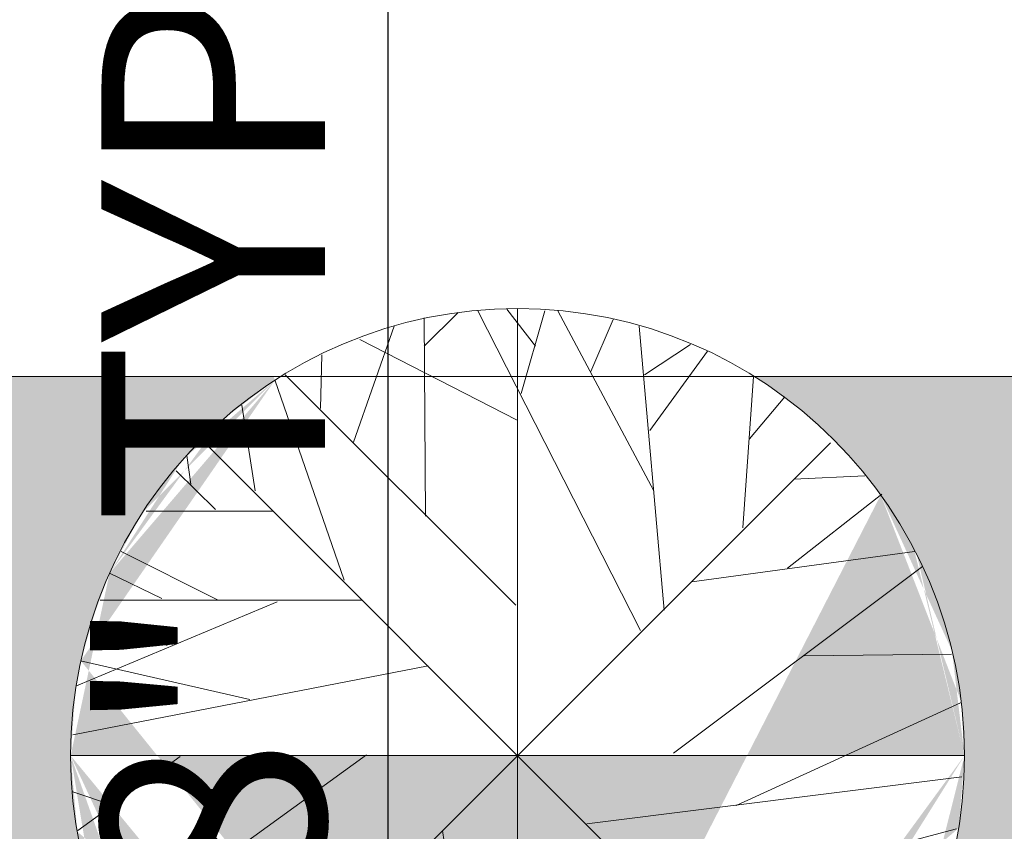
# Model space of a CAD drawing. Units: inches. Extents: x 459864 to 460310, y 324185 to 324787.
# Tile 60 of 112: x 460127 to 460154, y 324260 to 324282. Entities that reach past the tile are written whole.
import ezdxf

# ---------------------------------------------------------------- set-up
doc = ezdxf.new("R2010")
doc.units = ezdxf.units.IN
for name, color, linetype, lineweight in [('A-ANNO-DIMS', 2, 'Continuous', 18), ('L-PLNT', 3, 'Continuous', 13), ('L-SITE-PATT', 252, 'Continuous', 13)]:
    doc.layers.add(name, color=color, linetype=linetype, lineweight=lineweight)
doc.styles.get("Standard").update_dxf_attribs({"font": 'arial.ttf'})
doc.dimstyles.new('ISO-25', dxfattribs={"dimtxt": 6, "dimasz": 2.5, "dimexe": 1.25, "dimexo": 0.625, "dimtad": 1, "dimdec": 1, "dimlunit": 3, "dimtxsty": 'Standard', "dimcen": 2.5, "dimadec": 0, "dimazin": 0, "dimtfac": 1, "dimtdec": 1, "dimtmove": 0, "dimatfit": 3, "dimfxl": 1, "dimarcsym": 0})

# ---------------------------------------------------------------- blocks, each defined once
blk = doc.blocks.new('Tree - deciduous plan')
for p, q in [((-5.3205, 59.6806), (16.5105, 16.7963)), ((2.426, 54.9406), (-1.4472, 59.9056)), ((0, 59.9996), (0, -60)), ((0.4894, 48.6208), (3.6584, 59.6806)), ((18.2711, 35.5298), (5.419, 59.6806)), ((-12.5388, 54.9406), (-7.9613, 59.4546)), ((-12.3627, 32.1443), (-12.5388, 58.7776)), ((9.8203, 51.5549), (12.8133, 58.5516)), ((-22.0458, 42.0753), (-16.5881, 57.6486)), ((19.6795, 19.5047), (16.3344, 57.6486)), ((-21.1656, 55.8436), (-0.0388, 45.0094)), ((17.0387, 51.1035), (23.2006, 55.1666)), ((17.7429, 43.6552), (25.4894, 54.2636)), ((-26.4472, 46.5894), (-26.2712, 53.8116)), ((-32.6092, 50.4264), (-23.2782, 23.5674)), ((-31.2008, 51.1035), (-0.2149, 20.1818)), ((31.6513, 50.8778), (30.2429, 30.5643)), ((31.1232, 42.5267), (35.8767, 48.1693)), ((-37.0107, 47.0408), (-35.25, 35.5298)), ((-40.1797, 44.558), (-36.4825, 43.2038)), ((42, 42), (-42, -42)), ((42, -42), (-42, 42)), ((-43.8768, 36.4326), (-44.405, 40.2696)), ((-45.8134, 38.2383), (-40.5318, 33.0471)), ((37.1091, 37.1098), (46.6161, 37.5612)), ((36.2288, 25.1474), (48.9049, 35.0784)), ((-49.8627, 32.8214), (-32.7853, 32.8214)), ((-53.2078, 27.4044), (-40.1797, 20.859)), ((23.3767, 23.3417), (53.3063, 27.4044)), ((54.3626, 25.3731), (20.9119, 0.3198)), ((-54.7923, 24.4702), (-47.75, 21.0847)), ((-32.2571, 20.6333), (-59.1937, 9.348)), ((-56.0247, 20.859), (-20.8134, 20.859)), ((-57.081, 17.9248), (-47.0458, 14.7649)), ((38.5175, 13.4107), (58.2359, 13.6364)), ((-59.7219, 2.8025), (-12.0106, 12.0565)), ((-58.6656, 12.7336), (-35.9543, 7.5424)), ((29.3626, -6.6771), (59.4682, 7.091)), ((-54.6162, -24.7335), (-20.2853, 0.0941)), ((-60, 0), (60, 0)), ((-45.2853, -0.1316), (-59.0177, -10.0627)), ((9.2922, -9.1598), (59.6443, -2.8401)), ((-59.7219, -4.8714), (-54.2641, -6.6771)), ((-10.074, -10.0627), (-2.5036, -59.7178)), ((26.3697, -18.4138), (58.9401, -9.8369))]:
    blk.add_line(p, q)
blk.add_circle((0, 0), 60)
blk = doc.blocks.new('*D28')
at = {"layer": 'A-ANNO-DIMS', "color": 0, "lineweight": -2, "transparency": 16777216}
for p, q in [((460148.65, 324370.7), (460136.025, 324370.7)), ((460137.275, 324368.2), (460137.275, 324293.2)), ((460148.65, 324290.7), (460136.025, 324290.7)), ((460137.275, 324290.7), (460137.275, 324198.69))]:
    blk.add_line(p, q, dxfattribs=at)
at = {"layer": 'A-ANNO-DIMS', "color": 0, "transparency": 16777216}
for points in [[(460136.858, 324368.2), (460137.692, 324368.2), (460137.275, 324370.7)], [(460136.858, 324293.2), (460137.692, 324293.2), (460137.275, 324290.7)]]:
    blk.add_solid(points, dxfattribs=at)
at = {"layer": 'Defpoints', "color": 0, "transparency": 16777216}
for p in [(460149.275, 324370.7), (460137.275, 324290.7), (460149.275, 324290.7)]:
    blk.add_point(p, dxfattribs=at)
at = {"layer": 'A-ANNO-DIMS', "color": 0, "transparency": 16777216, "insert": (460133.363, 324243.445), "char_height": 6, "attachment_point": 5, "rotation": 90}
blk.add_mtext('QUEEN BED 6\'-8" TYP.', dxfattribs=at)

msp = doc.modelspace()

# ---------------------------------------------------------------- hatches: boundary and pattern name
at = {"layer": 'L-SITE-PATT'}
h = msp.add_hatch(dxfattribs=at)
h.set_pattern_fill('DOTS', color=256)
h.paths.add_polyline_path([(460269.804, 324283.483), (460247.115, 324283.483), (460121.929, 324283.483), (460121.929, 324252.473), (460117.429, 324252.473), (460110.124, 324252.473), (460110.124, 324243.287), (460080.83, 324243.287), (460080.83, 324252.473), (460061.115, 324252.473), (460061.115, 324251.882), (460077.909, 324251.882), (460077.909, 324199.483), (460080.83, 324199.483), (460080.83, 324207.553), (460110.124, 324207.553), (460110.124, 324199.483), (460110.813, 324199.483), (460262.115, 324199.483), (460269.804, 324199.483)], flags=17)
edge = h.paths.add_edge_path(flags=0)
edge.add_ellipse((460222.59, 324263.813), major_axis=(-8.485, 8.485), ratio=1, start_angle=405, end_angle=495, ccw=False)
edge.add_line((460214.821, 324254.66), (460214.832, 324254.666))
edge.add_ellipse((460222.59, 324263.813), major_axis=(-8.485, 8.485), ratio=1, start_angle=405, end_angle=495, ccw=False)
edge.add_line((460210.759, 324261.781), (460210.768, 324261.787))
edge.add_ellipse((460222.59, 324263.813), major_axis=(-8.485, 8.485), ratio=1, start_angle=405, end_angle=495, ccw=False)
edge.add_ellipse((460222.59, 324263.813), major_axis=(-8.485, 8.485), ratio=1, start_angle=392.754, end_angle=405, ccw=False)
edge.add_ellipse((460222.59, 324263.813), major_axis=(-8.485, 8.485), ratio=1, start_angle=380.9347, end_angle=392.754, ccw=False)
edge.add_line((460211.337, 324267.985), (460211.34, 324267.985))
edge.add_ellipse((460222.59, 324263.813), major_axis=(-8.485, 8.485), ratio=1, start_angle=380.9347, end_angle=392.754, ccw=False)
edge.add_ellipse((460222.59, 324263.813), major_axis=(-8.485, 8.485), ratio=1, start_angle=347.9015, end_angle=380.9347, ccw=False)
edge.add_ellipse((460222.59, 324263.813), major_axis=(-8.485, 8.485), ratio=1, start_angle=327.0619, end_angle=347.9015, ccw=False)
edge.add_ellipse((460222.59, 324263.813), major_axis=(-8.485, 8.485), ratio=1, start_angle=278.3246, end_angle=327.0619, ccw=False)
edge.add_line((460225.158, 324275.536), (460225.158, 324275.535))
edge.add_ellipse((460222.59, 324263.813), major_axis=(-8.485, 8.485), ratio=1, start_angle=278.3246, end_angle=327.0619, ccw=False)
edge.add_ellipse((460222.59, 324263.813), major_axis=(-8.485, 8.485), ratio=1, start_angle=260.6436, end_angle=278.3246, ccw=False)
edge.add_ellipse((460222.59, 324263.813), major_axis=(-8.485, 8.485), ratio=1, start_angle=225, end_angle=260.6436, ccw=False)
edge.add_line((460234.509, 324265.243), (460234.501, 324265.239))
edge.add_ellipse((460222.59, 324263.813), major_axis=(-8.485, 8.485), ratio=1, start_angle=225, end_angle=260.6436, ccw=False)
edge.add_ellipse((460222.59, 324263.813), major_axis=(-8.485, 8.485), ratio=1, start_angle=495, end_angle=585, ccw=False)
edge.add_line((460234.437, 324261.861), (460234.424, 324261.858))
edge.add_ellipse((460222.59, 324263.813), major_axis=(-8.485, 8.485), ratio=1, start_angle=495, end_angle=585, ccw=False)
edge.add_line((460227.95, 324253.067), (460227.946, 324253.083))
edge.add_ellipse((460222.59, 324263.813), major_axis=(-8.485, 8.485), ratio=1, start_angle=495, end_angle=585, ccw=False)
edge.add_line((460226.223, 324252.369), (460226.211, 324252.38))
edge.add_ellipse((460222.59, 324263.813), major_axis=(-8.485, 8.485), ratio=1, start_angle=495, end_angle=585, ccw=False)
h.paths.add_polyline_path([(460219.651, 324254.347), (460218.461, 324253.545), (460218.275, 324254.789), (460219.642, 324256.542), (460219.625, 324260.848), (460216.11, 324257.333), (460214.35, 324256.978), (460215.416, 324259.356), (460212.524, 324258.496), (460213.137, 324259.93), (460218.507, 324263.813), (460222.59, 324263.813), (460222.59, 324267.807), (460218.176, 324272.212), (460219.026, 324274.639), (460222.59, 324272.811), (460222.59, 324275.423), (460223.057, 324274.825), (460222.675, 324273.492), (460225.912, 324267.135), (460219.625, 324260.848)], flags=0)
edge = h.paths.add_edge_path(flags=0)
edge.add_ellipse((460194.576, 324264.046), major_axis=(-8.485, 8.485), ratio=1, start_angle=495, end_angle=585, ccw=False)
edge.add_line((460199.936, 324253.3), (460199.932, 324253.316))
edge.add_ellipse((460194.576, 324264.046), major_axis=(-8.485, 8.485), ratio=1, start_angle=495, end_angle=585, ccw=False)
edge.add_line((460198.208, 324252.603), (460198.196, 324252.613))
edge.add_ellipse((460194.576, 324264.046), major_axis=(-8.485, 8.485), ratio=1, start_angle=495, end_angle=585, ccw=False)
edge.add_ellipse((460194.576, 324264.046), major_axis=(-8.485, 8.485), ratio=1, start_angle=405, end_angle=495, ccw=False)
edge.add_line((460186.806, 324254.893), (460186.817, 324254.899))
edge.add_ellipse((460194.576, 324264.046), major_axis=(-8.485, 8.485), ratio=1, start_angle=405, end_angle=495, ccw=False)
edge.add_line((460182.744, 324262.014), (460182.753, 324262.02))
edge.add_ellipse((460194.576, 324264.046), major_axis=(-8.485, 8.485), ratio=1, start_angle=405, end_angle=495, ccw=False)
edge.add_ellipse((460194.576, 324264.046), major_axis=(-8.485, 8.485), ratio=1, start_angle=392.754, end_angle=405, ccw=False)
edge.add_ellipse((460194.576, 324264.046), major_axis=(-8.485, 8.485), ratio=1, start_angle=380.9347, end_angle=392.754, ccw=False)
edge.add_line((460183.323, 324268.218), (460183.326, 324268.218))
edge.add_ellipse((460194.576, 324264.046), major_axis=(-8.485, 8.485), ratio=1, start_angle=380.9347, end_angle=392.754, ccw=False)
edge.add_ellipse((460194.576, 324264.046), major_axis=(-8.485, 8.485), ratio=1, start_angle=347.9015, end_angle=380.9347, ccw=False)
edge.add_ellipse((460194.576, 324264.046), major_axis=(-8.485, 8.485), ratio=1, start_angle=327.0619, end_angle=347.9015, ccw=False)
edge.add_ellipse((460194.576, 324264.046), major_axis=(-8.485, 8.485), ratio=1, start_angle=278.3246, end_angle=327.0619, ccw=False)
edge.add_line((460197.144, 324275.769), (460197.143, 324275.768))
edge.add_ellipse((460194.576, 324264.046), major_axis=(-8.485, 8.485), ratio=1, start_angle=278.3246, end_angle=327.0619, ccw=False)
edge.add_ellipse((460194.576, 324264.046), major_axis=(-8.485, 8.485), ratio=1, start_angle=260.6436, end_angle=278.3246, ccw=False)
edge.add_ellipse((460194.576, 324264.046), major_axis=(-8.485, 8.485), ratio=1, start_angle=225, end_angle=260.6436, ccw=False)
edge.add_line((460206.494, 324265.476), (460206.487, 324265.473))
edge.add_ellipse((460194.576, 324264.046), major_axis=(-8.485, 8.485), ratio=1, start_angle=225, end_angle=260.6436, ccw=False)
edge.add_ellipse((460194.576, 324264.046), major_axis=(-8.485, 8.485), ratio=1, start_angle=495, end_angle=585, ccw=False)
edge.add_line((460206.422, 324262.094), (460206.409, 324262.091))
h.paths.add_polyline_path([(460191.61, 324261.081), (460191.637, 324254.58), (460190.447, 324253.778), (460190.261, 324255.023), (460191.628, 324256.775), (460191.61, 324261.081), (460188.096, 324257.566), (460186.335, 324257.211), (460187.402, 324259.589), (460184.509, 324258.729), (460185.123, 324260.163), (460190.493, 324264.046), (460194.576, 324264.046), (460194.576, 324268.04), (460190.161, 324272.446), (460191.011, 324274.872), (460194.576, 324273.044), (460194.576, 324275.657), (460195.043, 324275.058), (460194.661, 324273.725), (460197.897, 324267.368)], flags=0)
edge = h.paths.add_edge_path(flags=0)
edge.add_ellipse((460252.912, 324263.578), major_axis=(-8.485, 8.485), ratio=1, start_angle=405, end_angle=495, ccw=False)
edge.add_line((460241.081, 324261.545), (460241.089, 324261.551))
edge.add_ellipse((460252.912, 324263.578), major_axis=(-8.485, 8.485), ratio=1, start_angle=405, end_angle=495, ccw=False)
edge.add_ellipse((460252.912, 324263.578), major_axis=(-8.485, 8.485), ratio=1, start_angle=392.754, end_angle=405, ccw=False)
edge.add_ellipse((460252.912, 324263.578), major_axis=(-8.485, 8.485), ratio=1, start_angle=380.9347, end_angle=392.754, ccw=False)
edge.add_line((460241.659, 324267.749), (460241.662, 324267.749))
edge.add_ellipse((460252.912, 324263.578), major_axis=(-8.485, 8.485), ratio=1, start_angle=380.9347, end_angle=392.754, ccw=False)
edge.add_ellipse((460252.912, 324263.578), major_axis=(-8.485, 8.485), ratio=1, start_angle=347.9015, end_angle=380.9347, ccw=False)
edge.add_ellipse((460252.912, 324263.578), major_axis=(-8.485, 8.485), ratio=1, start_angle=327.0619, end_angle=347.9015, ccw=False)
edge.add_ellipse((460252.912, 324263.578), major_axis=(-8.485, 8.485), ratio=1, start_angle=278.3246, end_angle=327.0619, ccw=False)
edge.add_line((460255.48, 324275.3), (460255.479, 324275.299))
edge.add_ellipse((460252.912, 324263.578), major_axis=(-8.485, 8.485), ratio=1, start_angle=278.3246, end_angle=327.0619, ccw=False)
edge.add_ellipse((460252.912, 324263.578), major_axis=(-8.485, 8.485), ratio=1, start_angle=260.6436, end_angle=278.3246, ccw=False)
edge.add_ellipse((460252.912, 324263.578), major_axis=(-8.485, 8.485), ratio=1, start_angle=225, end_angle=260.6436, ccw=False)
edge.add_line((460264.83, 324265.007), (460264.823, 324265.004))
edge.add_ellipse((460252.912, 324263.578), major_axis=(-8.485, 8.485), ratio=1, start_angle=225, end_angle=260.6436, ccw=False)
edge.add_ellipse((460252.912, 324263.578), major_axis=(-8.485, 8.485), ratio=1, start_angle=495, end_angle=585, ccw=False)
edge.add_line((460264.758, 324261.626), (460264.745, 324261.622))
edge.add_ellipse((460252.912, 324263.578), major_axis=(-8.485, 8.485), ratio=1, start_angle=495, end_angle=585, ccw=False)
edge.add_line((460258.272, 324252.832), (460258.268, 324252.848))
edge.add_ellipse((460252.912, 324263.578), major_axis=(-8.485, 8.485), ratio=1, start_angle=495, end_angle=585, ccw=False)
edge.add_line((460256.545, 324252.134), (460256.533, 324252.144))
edge.add_ellipse((460252.912, 324263.578), major_axis=(-8.485, 8.485), ratio=1, start_angle=495, end_angle=585, ccw=False)
edge.add_ellipse((460252.912, 324263.578), major_axis=(-8.485, 8.485), ratio=1, start_angle=405, end_angle=495, ccw=False)
edge.add_line((460245.143, 324254.424), (460245.153, 324254.43))
h.paths.add_polyline_path([(460244.672, 324256.742), (460245.738, 324259.12), (460242.846, 324258.26), (460243.459, 324259.694), (460248.829, 324263.578), (460252.912, 324263.578), (460252.912, 324267.571), (460248.497, 324271.977), (460249.348, 324274.403), (460252.912, 324272.576), (460252.912, 324275.188), (460253.379, 324274.589), (460252.997, 324273.257), (460256.233, 324266.899), (460249.946, 324260.612), (460249.973, 324254.111), (460248.783, 324253.309), (460248.597, 324254.554), (460249.964, 324256.306), (460249.946, 324260.612), (460246.432, 324257.097)], flags=0)
edge = h.paths.add_edge_path(flags=0)
edge.add_ellipse((460167.439, 324262.833), major_axis=(-8.485, 8.485), ratio=1, start_angle=495, end_angle=585, ccw=False)
edge.add_line((460172.799, 324252.087), (460172.795, 324252.103))
edge.add_ellipse((460167.439, 324262.833), major_axis=(-8.485, 8.485), ratio=1, start_angle=495, end_angle=585, ccw=False)
edge.add_line((460171.071, 324251.389), (460171.059, 324251.399))
edge.add_ellipse((460167.439, 324262.833), major_axis=(-8.485, 8.485), ratio=1, start_angle=495, end_angle=585, ccw=False)
edge.add_ellipse((460167.439, 324262.833), major_axis=(-8.485, 8.485), ratio=1, start_angle=405, end_angle=495, ccw=False)
edge.add_line((460159.669, 324253.679), (460159.68, 324253.685))
edge.add_ellipse((460167.439, 324262.833), major_axis=(-8.485, 8.485), ratio=1, start_angle=405, end_angle=495, ccw=False)
edge.add_line((460155.607, 324260.8), (460155.616, 324260.806))
edge.add_ellipse((460167.439, 324262.833), major_axis=(-8.485, 8.485), ratio=1, start_angle=405, end_angle=495, ccw=False)
edge.add_ellipse((460167.439, 324262.833), major_axis=(-8.485, 8.485), ratio=1, start_angle=392.754, end_angle=405, ccw=False)
edge.add_ellipse((460167.439, 324262.833), major_axis=(-8.485, 8.485), ratio=1, start_angle=380.9347, end_angle=392.754, ccw=False)
edge.add_line((460156.185, 324267.005), (460156.189, 324267.005))
edge.add_ellipse((460167.439, 324262.833), major_axis=(-8.485, 8.485), ratio=1, start_angle=380.9347, end_angle=392.754, ccw=False)
edge.add_ellipse((460167.439, 324262.833), major_axis=(-8.485, 8.485), ratio=1, start_angle=347.9015, end_angle=380.9347, ccw=False)
edge.add_ellipse((460167.439, 324262.833), major_axis=(-8.485, 8.485), ratio=1, start_angle=327.0619, end_angle=347.9015, ccw=False)
edge.add_ellipse((460167.439, 324262.833), major_axis=(-8.485, 8.485), ratio=1, start_angle=278.3246, end_angle=327.0619, ccw=False)
edge.add_line((460170.007, 324274.556), (460170.006, 324274.554))
edge.add_ellipse((460167.439, 324262.833), major_axis=(-8.485, 8.485), ratio=1, start_angle=278.3246, end_angle=327.0619, ccw=False)
edge.add_ellipse((460167.439, 324262.833), major_axis=(-8.485, 8.485), ratio=1, start_angle=260.6436, end_angle=278.3246, ccw=False)
edge.add_ellipse((460167.439, 324262.833), major_axis=(-8.485, 8.485), ratio=1, start_angle=225, end_angle=260.6436, ccw=False)
edge.add_line((460179.357, 324264.262), (460179.35, 324264.259))
edge.add_ellipse((460167.439, 324262.833), major_axis=(-8.485, 8.485), ratio=1, start_angle=225, end_angle=260.6436, ccw=False)
edge.add_ellipse((460167.439, 324262.833), major_axis=(-8.485, 8.485), ratio=1, start_angle=495, end_angle=585, ccw=False)
edge.add_line((460179.285, 324260.881), (460179.272, 324260.877))
h.paths.add_polyline_path([(460164.473, 324259.867), (460164.5, 324253.366), (460163.31, 324252.565), (460163.124, 324253.809), (460164.491, 324255.561), (460164.473, 324259.867), (460160.958, 324256.353), (460159.198, 324255.998), (460160.265, 324258.375), (460157.372, 324257.515), (460157.986, 324258.949), (460163.356, 324262.833), (460167.439, 324262.833), (460167.439, 324266.826), (460163.024, 324271.232), (460163.874, 324273.659), (460167.439, 324271.831), (460167.439, 324274.443), (460167.905, 324273.844), (460167.524, 324272.512), (460170.76, 324266.154)], flags=0)
edge = h.paths.add_edge_path(flags=0)
edge.add_ellipse((460140.758, 324262.37), major_axis=(-8.485, 8.485), ratio=1, start_angle=495, end_angle=585, ccw=False)
edge.add_line((460146.118, 324251.624), (460146.114, 324251.639))
edge.add_ellipse((460140.758, 324262.37), major_axis=(-8.485, 8.485), ratio=1, start_angle=495, end_angle=585, ccw=False)
edge.add_line((460144.391, 324250.926), (460144.379, 324250.936))
edge.add_ellipse((460140.758, 324262.37), major_axis=(-8.485, 8.485), ratio=1, start_angle=495, end_angle=585, ccw=False)
edge.add_ellipse((460140.758, 324262.37), major_axis=(-8.485, 8.485), ratio=1, start_angle=405, end_angle=495, ccw=False)
edge.add_line((460132.989, 324253.216), (460132.999, 324253.222))
edge.add_ellipse((460140.758, 324262.37), major_axis=(-8.485, 8.485), ratio=1, start_angle=405, end_angle=495, ccw=False)
edge.add_line((460128.927, 324260.337), (460128.935, 324260.343))
edge.add_ellipse((460140.758, 324262.37), major_axis=(-8.485, 8.485), ratio=1, start_angle=405, end_angle=495, ccw=False)
edge.add_ellipse((460140.758, 324262.37), major_axis=(-8.485, 8.485), ratio=1, start_angle=392.754, end_angle=405, ccw=False)
edge.add_ellipse((460140.758, 324262.37), major_axis=(-8.485, 8.485), ratio=1, start_angle=380.9347, end_angle=392.754, ccw=False)
edge.add_line((460129.505, 324266.541), (460129.508, 324266.541))
edge.add_ellipse((460140.758, 324262.37), major_axis=(-8.485, 8.485), ratio=1, start_angle=380.9347, end_angle=392.754, ccw=False)
edge.add_ellipse((460140.758, 324262.37), major_axis=(-8.485, 8.485), ratio=1, start_angle=347.9015, end_angle=380.9347, ccw=False)
edge.add_ellipse((460140.758, 324262.37), major_axis=(-8.485, 8.485), ratio=1, start_angle=327.0619, end_angle=347.9015, ccw=False)
edge.add_ellipse((460140.758, 324262.37), major_axis=(-8.485, 8.485), ratio=1, start_angle=278.3246, end_angle=327.0619, ccw=False)
edge.add_line((460143.326, 324274.092), (460143.325, 324274.091))
edge.add_ellipse((460140.758, 324262.37), major_axis=(-8.485, 8.485), ratio=1, start_angle=278.3246, end_angle=327.0619, ccw=False)
edge.add_ellipse((460140.758, 324262.37), major_axis=(-8.485, 8.485), ratio=1, start_angle=260.6436, end_angle=278.3246, ccw=False)
edge.add_ellipse((460140.758, 324262.37), major_axis=(-8.485, 8.485), ratio=1, start_angle=225, end_angle=260.6436, ccw=False)
edge.add_line((460152.677, 324263.799), (460152.669, 324263.796))
edge.add_ellipse((460140.758, 324262.37), major_axis=(-8.485, 8.485), ratio=1, start_angle=225, end_angle=260.6436, ccw=False)
edge.add_ellipse((460140.758, 324262.37), major_axis=(-8.485, 8.485), ratio=1, start_angle=495, end_angle=585, ccw=False)
edge.add_line((460152.604, 324260.418), (460152.592, 324260.414))
h.paths.add_polyline_path([(460137.792, 324259.404), (460137.819, 324252.903), (460136.629, 324252.101), (460136.443, 324253.346), (460137.81, 324255.098), (460137.792, 324259.404), (460134.278, 324255.889), (460132.518, 324255.534), (460133.584, 324257.912), (460130.692, 324257.052), (460131.305, 324258.486), (460136.675, 324262.37), (460140.758, 324262.37), (460140.758, 324266.363), (460136.343, 324270.769), (460137.194, 324273.195), (460140.758, 324271.367), (460140.758, 324273.98), (460141.225, 324273.381), (460140.843, 324272.049), (460144.079, 324265.691)], flags=0)
h.paths.add_polyline_path([(460110.124, 324227.414), (460080.83, 324227.414), (460080.83, 324235.484), (460110.124, 324235.484)], flags=16)
h.paths.add_polyline_path([(460110.124, 324220.797), (460110.124, 324212.727), (460080.83, 324212.727), (460080.83, 324220.797)], flags=16)
h.paths.add_polyline_path([(460269.804, 324283.483), (460247.115, 324283.483), (460121.929, 324283.483), (460121.929, 324252.473), (460117.429, 324252.473), (460110.124, 324252.473), (460110.124, 324243.287), (460080.83, 324243.287), (460080.83, 324252.473), (460061.115, 324252.473), (460061.115, 324251.882), (460077.909, 324251.882), (460077.909, 324199.483), (460080.83, 324199.483), (460080.83, 324207.553), (460110.124, 324207.553), (460110.124, 324199.483), (460262.115, 324199.483), (460269.804, 324199.483)], flags=17)
h.paths.add_polyline_path([(460219.651, 324254.347), (460218.461, 324253.545), (460218.275, 324254.789), (460219.642, 324256.542), (460219.625, 324260.848), (460216.11, 324257.333), (460214.35, 324256.978), (460215.416, 324259.356), (460212.524, 324258.496), (460213.137, 324259.93), (460218.507, 324263.813), (460222.59, 324263.813), (460220.18, 324266.223), (460215.461, 324265.308), (460211.835, 324266.137), (460216.247, 324267.985), (460218.418, 324267.985), (460222.59, 324263.813), (460222.59, 324267.807), (460218.176, 324272.212), (460219.026, 324274.639), (460222.59, 324272.811), (460222.59, 324275.423), (460223.057, 324274.825), (460222.675, 324273.492), (460225.912, 324267.135), (460222.59, 324263.813), (460231.383, 324263.813), (460228.485, 324262.488), (460224.425, 324261.978), (460228.68, 324257.724), (460228.966, 324254.791), (460227.142, 324256.537), (460227.542, 324254.819), (460227.333, 324253.614), (460222.59, 324259.985), (460222.59, 324255.497), (460221.377, 324256.541), (460220.576, 324261.799), (460219.625, 324260.848)], flags=0)
h.paths.add_polyline_path([(460199.127, 324256.77), (460199.528, 324255.052), (460199.319, 324253.848), (460194.576, 324260.218), (460194.576, 324255.73), (460193.363, 324256.774), (460192.561, 324262.032), (460191.61, 324261.081), (460191.637, 324254.58), (460190.447, 324253.778), (460190.261, 324255.023), (460191.628, 324256.775), (460191.61, 324261.081), (460188.096, 324257.566), (460186.335, 324257.211), (460187.402, 324259.589), (460184.509, 324258.729), (460185.123, 324260.163), (460190.493, 324264.046), (460194.576, 324264.046), (460192.166, 324266.456), (460187.446, 324265.541), (460183.82, 324266.37), (460188.232, 324268.218), (460190.404, 324268.218), (460194.576, 324264.046), (460194.576, 324268.04), (460190.161, 324272.446), (460191.011, 324274.872), (460194.576, 324273.044), (460194.576, 324275.657), (460195.043, 324275.058), (460194.661, 324273.725), (460197.897, 324267.368), (460194.576, 324264.046), (460203.368, 324264.046), (460200.47, 324262.721), (460196.411, 324262.212), (460200.665, 324257.957), (460200.951, 324255.024)], flags=0)
h.paths.add_polyline_path([(460244.672, 324256.742), (460245.738, 324259.12), (460242.846, 324258.26), (460243.459, 324259.694), (460248.829, 324263.578), (460252.912, 324263.578), (460250.502, 324265.987), (460245.783, 324265.072), (460242.156, 324265.901), (460246.568, 324267.749), (460248.74, 324267.749), (460252.912, 324263.578), (460252.912, 324267.571), (460248.497, 324271.977), (460249.348, 324274.403), (460252.912, 324272.576), (460252.912, 324275.188), (460253.379, 324274.589), (460252.997, 324273.257), (460256.233, 324266.899), (460252.912, 324263.578), (460261.705, 324263.578), (460258.806, 324262.252), (460254.747, 324261.743), (460259.002, 324257.488), (460259.288, 324254.555), (460257.463, 324256.301), (460257.864, 324254.583), (460257.655, 324253.379), (460252.912, 324259.749), (460252.912, 324255.261), (460251.699, 324256.305), (460250.897, 324261.563), (460249.946, 324260.612), (460249.973, 324254.111), (460248.783, 324253.309), (460248.597, 324254.554), (460249.964, 324256.306), (460249.946, 324260.612), (460246.432, 324257.097)], flags=0)
h.paths.add_polyline_path([(460173.528, 324256.743), (460173.814, 324253.811), (460171.99, 324255.556), (460172.39, 324253.838), (460172.182, 324252.634), (460167.439, 324259.004), (460167.439, 324254.516), (460166.226, 324255.56), (460165.424, 324260.818), (460164.473, 324259.867), (460164.5, 324253.366), (460163.31, 324252.565), (460163.124, 324253.809), (460164.491, 324255.561), (460164.473, 324259.867), (460160.958, 324256.353), (460159.198, 324255.998), (460160.265, 324258.375), (460157.372, 324257.515), (460157.986, 324258.949), (460163.356, 324262.833), (460167.439, 324262.833), (460165.029, 324265.243), (460160.309, 324264.327), (460156.683, 324265.156), (460161.095, 324267.005), (460163.267, 324267.005), (460167.439, 324262.833), (460167.439, 324266.826), (460163.024, 324271.232), (460163.874, 324273.659), (460167.439, 324271.831), (460167.439, 324274.443), (460167.905, 324273.844), (460167.524, 324272.512), (460170.76, 324266.154), (460167.439, 324262.833), (460176.231, 324262.833), (460173.333, 324261.507), (460169.274, 324260.998)], flags=0)
h.paths.add_polyline_path([(460146.848, 324256.28), (460147.134, 324253.347), (460145.31, 324255.093), (460145.71, 324253.375), (460145.501, 324252.171), (460140.758, 324258.541), (460140.758, 324254.053), (460139.545, 324255.097), (460138.744, 324260.355), (460137.792, 324259.404), (460137.819, 324252.903), (460136.629, 324252.101), (460136.443, 324253.346), (460137.81, 324255.098), (460137.792, 324259.404), (460134.278, 324255.889), (460132.518, 324255.534), (460133.584, 324257.912), (460130.692, 324257.052), (460131.305, 324258.486), (460136.675, 324262.37), (460140.758, 324262.37), (460138.348, 324264.779), (460133.629, 324263.864), (460130.002, 324264.693), (460134.414, 324266.541), (460136.586, 324266.541), (460140.758, 324262.37), (460140.758, 324266.363), (460136.343, 324270.769), (460137.194, 324273.195), (460140.758, 324271.367), (460140.758, 324273.98), (460141.225, 324273.381), (460140.843, 324272.049), (460144.079, 324265.691), (460140.758, 324262.37), (460149.551, 324262.37), (460146.653, 324261.044), (460142.593, 324260.535)], flags=0)
edge = h.paths.add_edge_path()
edge.add_line((460269.804, 324272.549), (460260.881, 324272.549))
edge.add_ellipse((460252.912, 324263.578), major_axis=(-8.485, 8.485), ratio=1, start_angle=260.6436, end_angle=273.3846, ccw=False)
edge.add_line((460262.283, 324271.092), (460262.261, 324271.091))
edge.add_ellipse((460252.912, 324263.578), major_axis=(-8.485, 8.485), ratio=1, start_angle=260.6436, end_angle=273.3846, ccw=False)
edge.add_ellipse((460252.912, 324263.578), major_axis=(-8.485, 8.485), ratio=1, start_angle=225, end_angle=260.6436, ccw=False)
edge.add_line((460263.609, 324269.063), (460263.572, 324269.058))
edge.add_ellipse((460252.912, 324263.578), major_axis=(-8.485, 8.485), ratio=1, start_angle=225, end_angle=260.6436, ccw=False)
edge.add_line((460264.615, 324266.306), (460264.585, 324266.305))
edge.add_ellipse((460252.912, 324263.578), major_axis=(-8.485, 8.485), ratio=1, start_angle=225, end_angle=260.6436, ccw=False)
edge.add_line((460264.83, 324265.007), (460264.823, 324265.004))
edge.add_ellipse((460252.912, 324263.578), major_axis=(-8.485, 8.485), ratio=1, start_angle=225, end_angle=260.6436, ccw=False)
edge.add_ellipse((460252.912, 324263.578), major_axis=(-8.485, 8.485), ratio=1, start_angle=495, end_angle=585, ccw=False)
edge.add_line((460264.758, 324261.626), (460264.745, 324261.622))
edge.add_ellipse((460252.912, 324263.578), major_axis=(-8.485, 8.485), ratio=1, start_angle=495, end_angle=585, ccw=False)
edge.add_line((460263.442, 324257.739), (460263.389, 324257.779))
edge.add_ellipse((460252.912, 324263.578), major_axis=(-8.485, 8.485), ratio=1, start_angle=495, end_angle=585, ccw=False)
edge.add_line((460258.128, 324252.744), (460258.102, 324252.779))
edge.add_ellipse((460252.912, 324263.578), major_axis=(-8.485, 8.485), ratio=1, start_angle=495, end_angle=585, ccw=False)
edge.add_line((460256.545, 324252.134), (460256.533, 324252.144))
edge.add_ellipse((460252.912, 324263.578), major_axis=(-8.485, 8.485), ratio=1, start_angle=495, end_angle=585, ccw=False)
edge.add_ellipse((460252.912, 324263.578), major_axis=(-8.485, 8.485), ratio=1, start_angle=405, end_angle=495, ccw=False)
edge.add_line((460250.594, 324251.78), (460250.605, 324251.82))
edge.add_ellipse((460252.912, 324263.578), major_axis=(-8.485, 8.485), ratio=1, start_angle=405, end_angle=495, ccw=False)
edge.add_line((460245.143, 324254.424), (460245.153, 324254.43))
edge.add_ellipse((460252.912, 324263.578), major_axis=(-8.485, 8.485), ratio=1, start_angle=405, end_angle=495, ccw=False)
edge.add_line((460243.525, 324256.059), (460243.56, 324256.091))
edge.add_ellipse((460252.912, 324263.578), major_axis=(-8.485, 8.485), ratio=1, start_angle=405, end_angle=495, ccw=False)
edge.add_line((460241.44, 324259.893), (460241.522, 324259.896))
edge.add_ellipse((460252.912, 324263.578), major_axis=(-8.485, 8.485), ratio=1, start_angle=405, end_angle=495, ccw=False)
edge.add_line((460241.081, 324261.545), (460241.089, 324261.551))
edge.add_ellipse((460252.912, 324263.578), major_axis=(-8.485, 8.485), ratio=1, start_angle=405, end_angle=495, ccw=False)
edge.add_ellipse((460252.912, 324263.578), major_axis=(-8.485, 8.485), ratio=1, start_angle=392.754, end_angle=405, ccw=False)
edge.add_line((460241.05, 324265.438), (460241.063, 324265.443))
edge.add_ellipse((460252.912, 324263.578), major_axis=(-8.485, 8.485), ratio=1, start_angle=392.754, end_angle=405, ccw=False)
edge.add_ellipse((460252.912, 324263.578), major_axis=(-8.485, 8.485), ratio=1, start_angle=380.9347, end_angle=392.754, ccw=False)
edge.add_line((460241.452, 324267.176), (460241.469, 324267.171))
edge.add_ellipse((460252.912, 324263.578), major_axis=(-8.485, 8.485), ratio=1, start_angle=380.9347, end_angle=392.754, ccw=False)
edge.add_line((460241.659, 324267.749), (460241.662, 324267.749))
edge.add_ellipse((460252.912, 324263.578), major_axis=(-8.485, 8.485), ratio=1, start_angle=380.9347, end_angle=392.754, ccw=False)
edge.add_ellipse((460252.912, 324263.578), major_axis=(-8.485, 8.485), ratio=1, start_angle=356.6154, end_angle=380.9347, ccw=False)
edge.add_line((460244.88, 324272.488), (460244.713, 324272.549))
edge.add_line((460244.713, 324272.549), (460230.817, 324272.549))
edge.add_ellipse((460222.59, 324263.813), major_axis=(-8.485, 8.485), ratio=1, start_angle=260.6436, end_angle=271.7178, ccw=False)
edge.add_ellipse((460222.59, 324263.813), major_axis=(-8.485, 8.485), ratio=1, start_angle=225, end_angle=260.6436, ccw=False)
edge.add_line((460233.287, 324269.299), (460233.25, 324269.294))
edge.add_ellipse((460222.59, 324263.813), major_axis=(-8.485, 8.485), ratio=1, start_angle=225, end_angle=260.6436, ccw=False)
edge.add_line((460234.294, 324266.541), (460234.264, 324266.541))
edge.add_ellipse((460222.59, 324263.813), major_axis=(-8.485, 8.485), ratio=1, start_angle=225, end_angle=260.6436, ccw=False)
edge.add_line((460234.509, 324265.243), (460234.501, 324265.239))
edge.add_ellipse((460222.59, 324263.813), major_axis=(-8.485, 8.485), ratio=1, start_angle=225, end_angle=260.6436, ccw=False)
edge.add_ellipse((460222.59, 324263.813), major_axis=(-8.485, 8.485), ratio=1, start_angle=495, end_angle=585, ccw=False)
edge.add_line((460234.437, 324261.861), (460234.424, 324261.858))
edge.add_ellipse((460222.59, 324263.813), major_axis=(-8.485, 8.485), ratio=1, start_angle=495, end_angle=585, ccw=False)
edge.add_line((460233.121, 324257.975), (460233.068, 324258.015))
edge.add_ellipse((460222.59, 324263.813), major_axis=(-8.485, 8.485), ratio=1, start_angle=495, end_angle=585, ccw=False)
edge.add_line((460227.806, 324252.979), (460227.78, 324253.014))
edge.add_ellipse((460222.59, 324263.813), major_axis=(-8.485, 8.485), ratio=1, start_angle=495, end_angle=585, ccw=False)
edge.add_line((460226.223, 324252.369), (460226.211, 324252.38))
edge.add_ellipse((460222.59, 324263.813), major_axis=(-8.485, 8.485), ratio=1, start_angle=495, end_angle=585, ccw=False)
edge.add_ellipse((460222.59, 324263.813), major_axis=(-8.485, 8.485), ratio=1, start_angle=405, end_angle=495, ccw=False)
edge.add_line((460220.272, 324252.016), (460220.283, 324252.055))
edge.add_ellipse((460222.59, 324263.813), major_axis=(-8.485, 8.485), ratio=1, start_angle=405, end_angle=495, ccw=False)
edge.add_line((460214.821, 324254.66), (460214.832, 324254.666))
edge.add_ellipse((460222.59, 324263.813), major_axis=(-8.485, 8.485), ratio=1, start_angle=405, end_angle=495, ccw=False)
edge.add_line((460213.203, 324256.295), (460213.239, 324256.327))
edge.add_ellipse((460222.59, 324263.813), major_axis=(-8.485, 8.485), ratio=1, start_angle=405, end_angle=495, ccw=False)
edge.add_line((460211.118, 324260.128), (460211.201, 324260.131))
edge.add_ellipse((460222.59, 324263.813), major_axis=(-8.485, 8.485), ratio=1, start_angle=405, end_angle=495, ccw=False)
edge.add_line((460210.759, 324261.781), (460210.768, 324261.787))
edge.add_ellipse((460222.59, 324263.813), major_axis=(-8.485, 8.485), ratio=1, start_angle=405, end_angle=495, ccw=False)
edge.add_ellipse((460222.59, 324263.813), major_axis=(-8.485, 8.485), ratio=1, start_angle=392.754, end_angle=405, ccw=False)
edge.add_line((460210.729, 324265.673), (460210.741, 324265.678))
edge.add_ellipse((460222.59, 324263.813), major_axis=(-8.485, 8.485), ratio=1, start_angle=392.754, end_angle=405, ccw=False)
edge.add_ellipse((460222.59, 324263.813), major_axis=(-8.485, 8.485), ratio=1, start_angle=380.9347, end_angle=392.754, ccw=False)
edge.add_line((460211.13, 324267.412), (460211.147, 324267.407))
edge.add_ellipse((460222.59, 324263.813), major_axis=(-8.485, 8.485), ratio=1, start_angle=380.9347, end_angle=392.754, ccw=False)
edge.add_line((460211.337, 324267.985), (460211.34, 324267.985))
edge.add_ellipse((460222.59, 324263.813), major_axis=(-8.485, 8.485), ratio=1, start_angle=380.9347, end_angle=392.754, ccw=False)
edge.add_ellipse((460222.59, 324263.813), major_axis=(-8.485, 8.485), ratio=1, start_angle=358.2822, end_angle=380.9347, ccw=False)
edge.add_line((460213.705, 324271.902), (460213.709, 324271.869))
edge.add_ellipse((460222.59, 324263.813), major_axis=(-8.485, 8.485), ratio=1, start_angle=358.2822, end_angle=380.9347, ccw=False)
edge.add_line((460214.363, 324272.549), (460203.078, 324272.549))
edge.add_line((460203.078, 324272.549), (460203.06, 324272.531))
edge.add_ellipse((460194.576, 324264.046), major_axis=(-8.485, 8.485), ratio=1, start_angle=260.6436, end_angle=270.1168, ccw=False)
edge.add_line((460203.957, 324271.561), (460203.921, 324271.56))
edge.add_ellipse((460194.576, 324264.046), major_axis=(-8.485, 8.485), ratio=1, start_angle=260.6436, end_angle=270.1168, ccw=False)
edge.add_ellipse((460194.576, 324264.046), major_axis=(-8.485, 8.485), ratio=1, start_angle=225, end_angle=260.6436, ccw=False)
edge.add_line((460205.272, 324269.532), (460205.235, 324269.527))
edge.add_ellipse((460194.576, 324264.046), major_axis=(-8.485, 8.485), ratio=1, start_angle=225, end_angle=260.6436, ccw=False)
edge.add_line((460206.279, 324266.774), (460206.249, 324266.774))
edge.add_ellipse((460194.576, 324264.046), major_axis=(-8.485, 8.485), ratio=1, start_angle=225, end_angle=260.6436, ccw=False)
edge.add_line((460206.494, 324265.476), (460206.487, 324265.473))
edge.add_ellipse((460194.576, 324264.046), major_axis=(-8.485, 8.485), ratio=1, start_angle=225, end_angle=260.6436, ccw=False)
edge.add_ellipse((460194.576, 324264.046), major_axis=(-8.485, 8.485), ratio=1, start_angle=495, end_angle=585, ccw=False)
edge.add_line((460206.422, 324262.094), (460206.409, 324262.091))
edge.add_ellipse((460194.576, 324264.046), major_axis=(-8.485, 8.485), ratio=1, start_angle=495, end_angle=585, ccw=False)
edge.add_line((460205.106, 324258.208), (460205.053, 324258.248))
edge.add_ellipse((460194.576, 324264.046), major_axis=(-8.485, 8.485), ratio=1, start_angle=495, end_angle=585, ccw=False)
edge.add_line((460199.792, 324253.212), (460199.766, 324253.248))
edge.add_ellipse((460194.576, 324264.046), major_axis=(-8.485, 8.485), ratio=1, start_angle=495, end_angle=585, ccw=False)
edge.add_line((460198.208, 324252.603), (460198.196, 324252.613))
edge.add_ellipse((460194.576, 324264.046), major_axis=(-8.485, 8.485), ratio=1, start_angle=495, end_angle=585, ccw=False)
edge.add_ellipse((460194.576, 324264.046), major_axis=(-8.485, 8.485), ratio=1, start_angle=405, end_angle=495, ccw=False)
edge.add_line((460192.258, 324252.249), (460192.268, 324252.289))
edge.add_ellipse((460194.576, 324264.046), major_axis=(-8.485, 8.485), ratio=1, start_angle=405, end_angle=495, ccw=False)
edge.add_line((460186.806, 324254.893), (460186.817, 324254.899))
edge.add_ellipse((460194.576, 324264.046), major_axis=(-8.485, 8.485), ratio=1, start_angle=405, end_angle=495, ccw=False)
edge.add_line((460185.188, 324256.528), (460185.224, 324256.56))
edge.add_ellipse((460194.576, 324264.046), major_axis=(-8.485, 8.485), ratio=1, start_angle=405, end_angle=495, ccw=False)
edge.add_line((460183.104, 324260.362), (460183.186, 324260.365))
edge.add_ellipse((460194.576, 324264.046), major_axis=(-8.485, 8.485), ratio=1, start_angle=405, end_angle=495, ccw=False)
edge.add_line((460182.744, 324262.014), (460182.753, 324262.02))
edge.add_ellipse((460194.576, 324264.046), major_axis=(-8.485, 8.485), ratio=1, start_angle=405, end_angle=495, ccw=False)
edge.add_ellipse((460194.576, 324264.046), major_axis=(-8.485, 8.485), ratio=1, start_angle=392.754, end_angle=405, ccw=False)
edge.add_line((460182.714, 324265.906), (460182.726, 324265.912))
edge.add_ellipse((460194.576, 324264.046), major_axis=(-8.485, 8.485), ratio=1, start_angle=392.754, end_angle=405, ccw=False)
edge.add_ellipse((460194.576, 324264.046), major_axis=(-8.485, 8.485), ratio=1, start_angle=380.9347, end_angle=392.754, ccw=False)
edge.add_line((460183.116, 324267.645), (460183.133, 324267.64))
edge.add_ellipse((460194.576, 324264.046), major_axis=(-8.485, 8.485), ratio=1, start_angle=380.9347, end_angle=392.754, ccw=False)
edge.add_line((460183.323, 324268.218), (460183.326, 324268.218))
edge.add_ellipse((460194.576, 324264.046), major_axis=(-8.485, 8.485), ratio=1, start_angle=380.9347, end_angle=392.754, ccw=False)
edge.add_ellipse((460194.576, 324264.046), major_axis=(-8.485, 8.485), ratio=1, start_angle=359.8832, end_angle=380.9347, ccw=False)
edge.add_line((460184.491, 324270.611), (460184.553, 324270.611))
edge.add_ellipse((460194.576, 324264.046), major_axis=(-8.485, 8.485), ratio=1, start_angle=359.8832, end_angle=380.9347, ccw=False)
edge.add_line((460185.346, 324271.76), (460185.379, 324271.728))
edge.add_ellipse((460194.576, 324264.046), major_axis=(-8.485, 8.485), ratio=1, start_angle=359.8832, end_angle=380.9347, ccw=False)
edge.add_line((460185.697, 324272.086), (460185.633, 324272.549))
edge.add_line((460185.633, 324272.549), (460174.683, 324272.549))
edge.add_line((460174.683, 324272.549), (460174.606, 324272.457))
edge.add_ellipse((460167.439, 324262.833), major_axis=(-8.485, 8.485), ratio=1, start_angle=260.6436, end_angle=278.3246, ccw=False)
edge.add_ellipse((460167.439, 324262.833), major_axis=(-8.485, 8.485), ratio=1, start_angle=225, end_angle=260.6436, ccw=False)
edge.add_line((460178.135, 324268.318), (460178.098, 324268.313))
edge.add_ellipse((460167.439, 324262.833), major_axis=(-8.485, 8.485), ratio=1, start_angle=225, end_angle=260.6436, ccw=False)
edge.add_line((460179.142, 324265.561), (460179.112, 324265.56))
edge.add_ellipse((460167.439, 324262.833), major_axis=(-8.485, 8.485), ratio=1, start_angle=225, end_angle=260.6436, ccw=False)
edge.add_line((460179.357, 324264.262), (460179.35, 324264.259))
edge.add_ellipse((460167.439, 324262.833), major_axis=(-8.485, 8.485), ratio=1, start_angle=225, end_angle=260.6436, ccw=False)
edge.add_ellipse((460167.439, 324262.833), major_axis=(-8.485, 8.485), ratio=1, start_angle=495, end_angle=585, ccw=False)
edge.add_line((460179.285, 324260.881), (460179.272, 324260.877))
edge.add_ellipse((460167.439, 324262.833), major_axis=(-8.485, 8.485), ratio=1, start_angle=495, end_angle=585, ccw=False)
edge.add_line((460177.969, 324256.994), (460177.916, 324257.034))
edge.add_ellipse((460167.439, 324262.833), major_axis=(-8.485, 8.485), ratio=1, start_angle=495, end_angle=585, ccw=False)
edge.add_line((460172.655, 324251.999), (460172.629, 324252.034))
edge.add_ellipse((460167.439, 324262.833), major_axis=(-8.485, 8.485), ratio=1, start_angle=495, end_angle=585, ccw=False)
edge.add_line((460171.071, 324251.389), (460171.059, 324251.399))
edge.add_ellipse((460167.439, 324262.833), major_axis=(-8.485, 8.485), ratio=1, start_angle=495, end_angle=585, ccw=False)
edge.add_ellipse((460167.439, 324262.833), major_axis=(-8.485, 8.485), ratio=1, start_angle=405, end_angle=495, ccw=False)
edge.add_line((460165.121, 324251.036), (460165.131, 324251.075))
edge.add_ellipse((460167.439, 324262.833), major_axis=(-8.485, 8.485), ratio=1, start_angle=405, end_angle=495, ccw=False)
edge.add_line((460159.669, 324253.679), (460159.68, 324253.685))
edge.add_ellipse((460167.439, 324262.833), major_axis=(-8.485, 8.485), ratio=1, start_angle=405, end_angle=495, ccw=False)
edge.add_line((460158.051, 324255.314), (460158.087, 324255.347))
edge.add_ellipse((460167.439, 324262.833), major_axis=(-8.485, 8.485), ratio=1, start_angle=405, end_angle=495, ccw=False)
edge.add_line((460155.967, 324259.148), (460156.049, 324259.151))
edge.add_ellipse((460167.439, 324262.833), major_axis=(-8.485, 8.485), ratio=1, start_angle=405, end_angle=495, ccw=False)
edge.add_line((460155.607, 324260.8), (460155.616, 324260.806))
edge.add_ellipse((460167.439, 324262.833), major_axis=(-8.485, 8.485), ratio=1, start_angle=405, end_angle=495, ccw=False)
edge.add_ellipse((460167.439, 324262.833), major_axis=(-8.485, 8.485), ratio=1, start_angle=392.754, end_angle=405, ccw=False)
edge.add_line((460155.577, 324264.693), (460155.589, 324264.698))
edge.add_ellipse((460167.439, 324262.833), major_axis=(-8.485, 8.485), ratio=1, start_angle=392.754, end_angle=405, ccw=False)
edge.add_ellipse((460167.439, 324262.833), major_axis=(-8.485, 8.485), ratio=1, start_angle=380.9347, end_angle=392.754, ccw=False)
edge.add_line((460155.979, 324266.432), (460155.996, 324266.426))
edge.add_ellipse((460167.439, 324262.833), major_axis=(-8.485, 8.485), ratio=1, start_angle=380.9347, end_angle=392.754, ccw=False)
edge.add_line((460156.185, 324267.005), (460156.189, 324267.005))
edge.add_ellipse((460167.439, 324262.833), major_axis=(-8.485, 8.485), ratio=1, start_angle=380.9347, end_angle=392.754, ccw=False)
edge.add_ellipse((460167.439, 324262.833), major_axis=(-8.485, 8.485), ratio=1, start_angle=350.9345, end_angle=380.9347, ccw=False)
edge.add_line((460157.363, 324269.397), (460157.414, 324269.397))
edge.add_ellipse((460167.439, 324262.833), major_axis=(-8.485, 8.485), ratio=1, start_angle=350.9345, end_angle=380.9347, ccw=False)
edge.add_line((460158.221, 324270.535), (460158.236, 324270.519))
edge.add_ellipse((460167.439, 324262.833), major_axis=(-8.485, 8.485), ratio=1, start_angle=350.9345, end_angle=380.9347, ccw=False)
edge.add_line((460159.379, 324271.753), (460159.419, 324271.738))
edge.add_ellipse((460167.439, 324262.833), major_axis=(-8.485, 8.485), ratio=1, start_angle=350.9345, end_angle=380.9347, ccw=False)
edge.add_line((460160.396, 324272.549), (460147.112, 324272.549))
edge.add_ellipse((460140.758, 324262.37), major_axis=(-8.485, 8.485), ratio=1, start_angle=278.3246, end_angle=283.0261, ccw=False)
edge.add_ellipse((460140.758, 324262.37), major_axis=(-8.485, 8.485), ratio=1, start_angle=260.6436, end_angle=278.3246, ccw=False)
edge.add_ellipse((460140.758, 324262.37), major_axis=(-8.485, 8.485), ratio=1, start_angle=225, end_angle=260.6436, ccw=False)
edge.add_line((460151.455, 324267.855), (460151.418, 324267.85))
edge.add_ellipse((460140.758, 324262.37), major_axis=(-8.485, 8.485), ratio=1, start_angle=225, end_angle=260.6436, ccw=False)
edge.add_line((460152.462, 324265.098), (460152.431, 324265.097))
edge.add_ellipse((460140.758, 324262.37), major_axis=(-8.485, 8.485), ratio=1, start_angle=225, end_angle=260.6436, ccw=False)
edge.add_line((460152.677, 324263.799), (460152.669, 324263.796))
edge.add_ellipse((460140.758, 324262.37), major_axis=(-8.485, 8.485), ratio=1, start_angle=225, end_angle=260.6436, ccw=False)
edge.add_ellipse((460140.758, 324262.37), major_axis=(-8.485, 8.485), ratio=1, start_angle=495, end_angle=585, ccw=False)
edge.add_line((460152.604, 324260.418), (460152.592, 324260.414))
edge.add_ellipse((460140.758, 324262.37), major_axis=(-8.485, 8.485), ratio=1, start_angle=495, end_angle=585, ccw=False)
edge.add_line((460151.288, 324256.531), (460151.235, 324256.571))
edge.add_ellipse((460140.758, 324262.37), major_axis=(-8.485, 8.485), ratio=1, start_angle=495, end_angle=585, ccw=False)
edge.add_line((460145.974, 324251.535), (460145.948, 324251.571))
edge.add_ellipse((460140.758, 324262.37), major_axis=(-8.485, 8.485), ratio=1, start_angle=495, end_angle=585, ccw=False)
edge.add_line((460144.391, 324250.926), (460144.379, 324250.936))
edge.add_ellipse((460140.758, 324262.37), major_axis=(-8.485, 8.485), ratio=1, start_angle=495, end_angle=585, ccw=False)
edge.add_ellipse((460140.758, 324262.37), major_axis=(-8.485, 8.485), ratio=1, start_angle=405, end_angle=495, ccw=False)
edge.add_line((460138.44, 324250.572), (460138.451, 324250.612))
edge.add_ellipse((460140.758, 324262.37), major_axis=(-8.485, 8.485), ratio=1, start_angle=405, end_angle=495, ccw=False)
edge.add_line((460132.989, 324253.216), (460132.999, 324253.222))
edge.add_ellipse((460140.758, 324262.37), major_axis=(-8.485, 8.485), ratio=1, start_angle=405, end_angle=495, ccw=False)
edge.add_line((460131.371, 324254.851), (460131.406, 324254.883))
edge.add_ellipse((460140.758, 324262.37), major_axis=(-8.485, 8.485), ratio=1, start_angle=405, end_angle=495, ccw=False)
edge.add_line((460129.286, 324258.685), (460129.369, 324258.688))
edge.add_ellipse((460140.758, 324262.37), major_axis=(-8.485, 8.485), ratio=1, start_angle=405, end_angle=495, ccw=False)
edge.add_line((460128.927, 324260.337), (460128.935, 324260.343))
edge.add_ellipse((460140.758, 324262.37), major_axis=(-8.485, 8.485), ratio=1, start_angle=405, end_angle=495, ccw=False)
edge.add_ellipse((460140.758, 324262.37), major_axis=(-8.485, 8.485), ratio=1, start_angle=392.754, end_angle=405, ccw=False)
edge.add_line((460128.896, 324264.23), (460128.909, 324264.235))
edge.add_ellipse((460140.758, 324262.37), major_axis=(-8.485, 8.485), ratio=1, start_angle=392.754, end_angle=405, ccw=False)
edge.add_ellipse((460140.758, 324262.37), major_axis=(-8.485, 8.485), ratio=1, start_angle=380.9347, end_angle=392.754, ccw=False)
edge.add_line((460129.298, 324265.968), (460129.315, 324265.963))
edge.add_ellipse((460140.758, 324262.37), major_axis=(-8.485, 8.485), ratio=1, start_angle=380.9347, end_angle=392.754, ccw=False)
edge.add_line((460129.505, 324266.541), (460129.508, 324266.541))
edge.add_ellipse((460140.758, 324262.37), major_axis=(-8.485, 8.485), ratio=1, start_angle=380.9347, end_angle=392.754, ccw=False)
edge.add_ellipse((460140.758, 324262.37), major_axis=(-8.485, 8.485), ratio=1, start_angle=347.9015, end_angle=380.9347, ccw=False)
edge.add_line((460130.697, 324268.934), (460130.727, 324268.934))
edge.add_ellipse((460140.758, 324262.37), major_axis=(-8.485, 8.485), ratio=1, start_angle=347.9015, end_angle=380.9347, ccw=False)
edge.add_line((460131.869, 324270.48), (460131.879, 324270.413))
edge.add_ellipse((460140.758, 324262.37), major_axis=(-8.485, 8.485), ratio=1, start_angle=347.9015, end_angle=380.9347, ccw=False)
edge.add_line((460132.734, 324271.277), (460132.705, 324271.287))
edge.add_ellipse((460140.758, 324262.37), major_axis=(-8.485, 8.485), ratio=1, start_angle=347.9015, end_angle=380.9347, ccw=False)
edge.add_line((460134.24, 324272.445), (460134.204, 324272.549))
edge.add_line((460134.204, 324272.549), (460121.929, 324272.549))
edge.add_line((460121.929, 324272.549), (460121.929, 324252.473))
edge.add_line((460121.929, 324252.473), (460117.429, 324252.473))
edge.add_line((460117.429, 324252.473), (460110.124, 324252.473))
edge.add_line((460110.124, 324252.473), (460110.124, 324243.287))
edge.add_line((460110.124, 324243.287), (460080.83, 324243.287))
edge.add_line((460080.83, 324243.287), (460080.83, 324252.473))
edge.add_line((460080.83, 324252.473), (460061.115, 324252.473))
edge.add_line((460061.115, 324252.473), (460061.115, 324251.882))
edge.add_line((460061.115, 324251.882), (460077.909, 324251.882))
edge.add_line((460077.909, 324251.882), (460077.909, 324199.483))
edge.add_line((460077.909, 324199.483), (460080.83, 324199.483))
edge.add_line((460080.83, 324199.483), (460080.83, 324207.553))
edge.add_line((460080.83, 324207.553), (460110.124, 324207.553))
edge.add_line((460110.124, 324207.553), (460110.124, 324199.483))
edge.add_line((460110.124, 324199.483), (460110.813, 324199.483))
edge.add_line((460110.813, 324199.483), (460262.115, 324199.483))
edge.add_line((460262.115, 324199.483), (460269.804, 324199.483))
edge.add_line((460269.804, 324199.483), (460269.804, 324272.549))

# ---------------------------------------------------------------- linework, layer by layer
at = {"layer": 'L-PLNT'}
msp.add_line((460121.929, 324272.549), (460269.804, 324272.549), dxfattribs=at)

# ---------------------------------------------------------------- block references
at = {"layer": 'L-PLNT', "xscale": 0.2, "yscale": 0.2}
msp.add_blockref('Tree - deciduous plan', (460140.758, 324262.37), dxfattribs=at)

# ---------------------------------------------------------------- dimensions: what is measured, and where the dimension line sits
at = {"layer": 'A-ANNO-DIMS'}
dim = msp.add_linear_dim(base=(460137.275, 324290.7), p1=(460149.275, 324370.7), p2=(460149.275, 324290.7), angle=270, text='QUEEN BED <> TYP.', dimstyle='ISO-25', override={"dimdec": 1, "dimlfac": 1, "dimrnd": 0, "dimzin": 1, "dimdsep": 46, "dimlunit": 4, "dimfrac": 2}, dxfattribs=at)
dim.commit()
dim.dimension.update_dxf_attribs({"geometry": '*D28', "text_midpoint": (460133.363, 324243.445)})

doc.saveas('drawing.dxf')
